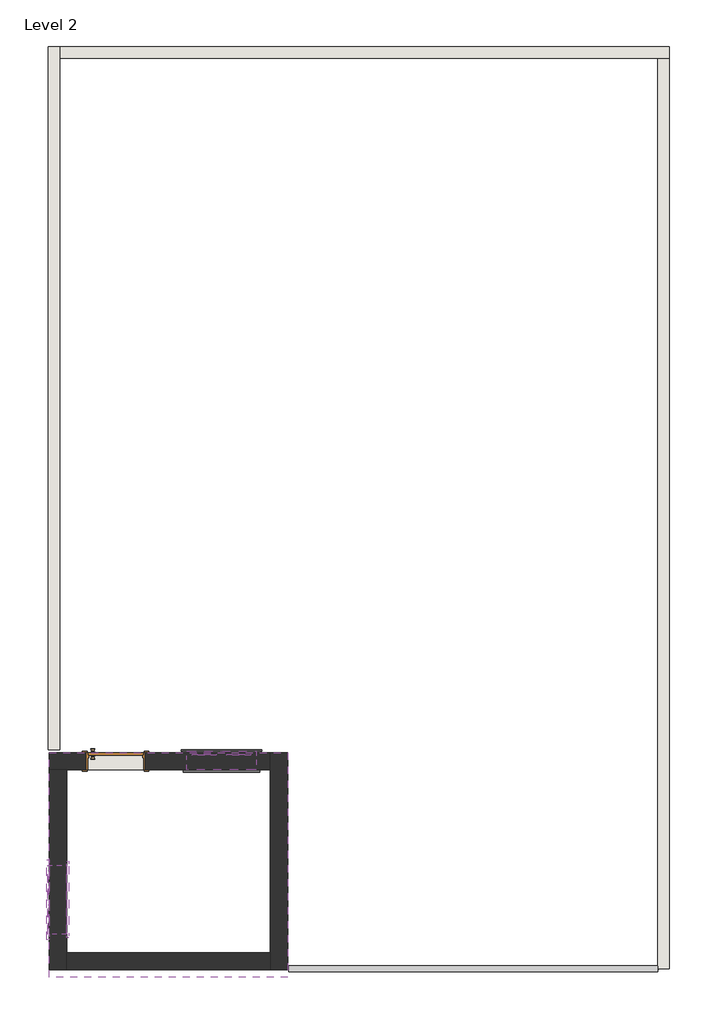
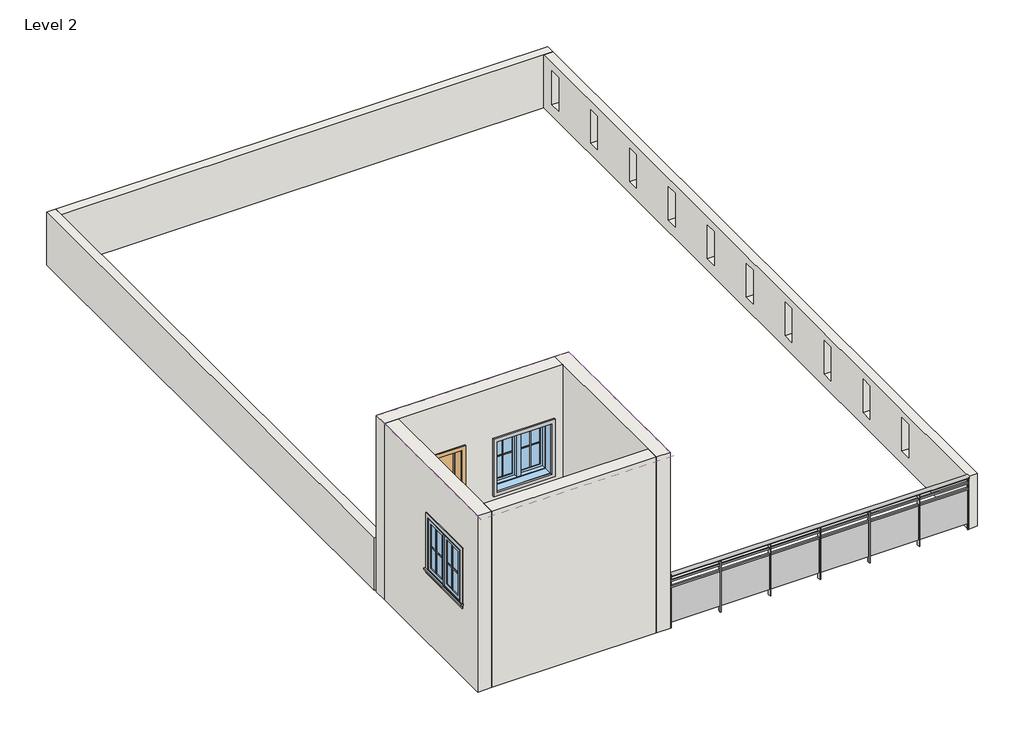
# One storey: 8 proxies, 7 walls, 2 windows, 1 covering, 1 door, 1 railing.
"""IFC4 building model written with IfcOpenShell, lengths in millimetres."""

from ifc_helpers import new_model, si_unit, point, frame, origin, place, context, project, spatial, polyline, ellipse_curve, trimmed, outline, extrude, faceted_brep, transform, mapped, element, save
from ifc_brep_helpers import plane_surface, extruded_surface, advanced_brep
from components import m_muntin_pattern_2x2_m_muntin_pattern_2x2_55460d9e, m_muntin_pattern_2x2_m_muntin_pattern_2x2_a9b7b7a9, m_trim_window_exterior_flat_with_sill_8fa486dc, m_trim_window_interior_flat_picture_frame_b6dd03a6, m_door_interior_single_flush_panel_wood_m_door_interior_542f8053, m_window_casement_double_914_x_900mm_7ae2d64b

model = new_model("IFC4")

# Units and contexts
model_context = context("Model", 3, world=origin())
ifc_project = project(units=[si_unit("LENGTHUNIT", "METRE", prefix="MILLI")], contexts=[model_context])

# Site, building, storey
site = spatial("IfcSite", under=ifc_project)
building = spatial("IfcBuilding", under=site)
storey = spatial("IfcBuildingStorey", under=building, Name="Level 2", Elevation=3048.0)

# Proxies
placement = place(None, origin())
m_muntin_pattern_2x2_m_muntin_pattern_2x2_shape = m_muntin_pattern_2x2_m_muntin_pattern_2x2_55460d9e(model_context)
element("IfcBuildingElementProxy", 1, Name="M_Muntin Pattern_2x2 : M_Muntin Pattern_2x2", ObjectType="M_Muntin Pattern_2x2 : M_Muntin Pattern_2x2", at=placement, inside=storey, context=model_context, shape_type="MappedRepresentation", body=[
    mapped(m_muntin_pattern_2x2_m_muntin_pattern_2x2_shape, transform((-3709.2004317, -3162.8938563, 4343.0929106), x_axis=(1.0, 0.0, 0.0), y_axis=(0.0, 1.0, 0.0), z_axis=(0.0, 0.0, 1.0))),
])
element("IfcBuildingElementProxy", 2, Name="M_Muntin Pattern_2x2 : M_Muntin Pattern_2x2", ObjectType="M_Muntin Pattern_2x2 : M_Muntin Pattern_2x2", at=placement, inside=storey, context=model_context, shape_type="MappedRepresentation", body=[
    mapped(m_muntin_pattern_2x2_m_muntin_pattern_2x2_shape, transform((-5746.7629317, -5323.4813563, 4402.5622211), x_axis=(0.0, 1.0, 0.0), y_axis=(-1.0, 0.0, 0.0), z_axis=(0.0, 0.0, 1.0))),
])
m_muntin_pattern_2x2_m_muntin_pattern_2x2_2_shape = m_muntin_pattern_2x2_m_muntin_pattern_2x2_a9b7b7a9(model_context)
element("IfcBuildingElementProxy", 3, Name="M_Muntin Pattern_2x2 : M_Muntin Pattern_2x2", ObjectType="M_Muntin Pattern_2x2 : M_Muntin Pattern_2x2", at=placement, inside=storey, context=model_context, shape_type="MappedRepresentation", body=[
    mapped(m_muntin_pattern_2x2_m_muntin_pattern_2x2_2_shape, transform((-3255.1754317, -3162.8938563, 4343.0929106), x_axis=(-1.0, 0.0, 0.0), y_axis=(0.0, -1.0, 0.0), z_axis=(0.0, 0.0, 1.0))),
])
element("IfcBuildingElementProxy", 4, Name="M_Muntin Pattern_2x2 : M_Muntin Pattern_2x2", ObjectType="M_Muntin Pattern_2x2 : M_Muntin Pattern_2x2", at=placement, inside=storey, context=model_context, shape_type="MappedRepresentation", body=[
    mapped(m_muntin_pattern_2x2_m_muntin_pattern_2x2_2_shape, transform((-5746.7629317, -4869.4563563, 4402.5622211), x_axis=(0.0, -1.0, 0.0), y_axis=(1.0, 0.0, 0.0), z_axis=(0.0, 0.0, 1.0))),
])
m_trim_window_exterior_flat_with_sill_shape = m_trim_window_exterior_flat_with_sill_8fa486dc(model_context)
element("IfcBuildingElementProxy", 5, Name="M_Trim-Window-Exterior-Flat : with Sill", ObjectType="M_Trim-Window-Exterior-Flat : with Sill", at=placement, inside=storey, context=model_context, shape_type="MappedRepresentation", body=[
    mapped(m_trim_window_exterior_flat_with_sill_shape, transform((-3482.1879317, -3153.3688563, 5173.2429106), x_axis=(-1.0, 0.0, 0.0), y_axis=(0.0, 0.0, 1.0), z_axis=(0.0, 1.0, 0.0))),
])
element("IfcBuildingElementProxy", 6, Name="M_Trim-Window-Exterior-Flat : with Sill", ObjectType="M_Trim-Window-Exterior-Flat : with Sill", at=placement, inside=storey, context=model_context, shape_type="MappedRepresentation", body=[
    mapped(m_trim_window_exterior_flat_with_sill_shape, transform((-5756.2879317, -5096.4688563, 5232.7122211), x_axis=(0.0, -1.0, 0.0), y_axis=(0.0, 0.0, 1.0), z_axis=(-1.0, 0.0, 0.0))),
])
m_trim_window_interior_flat_picture_frame_shape = m_trim_window_interior_flat_picture_frame_b6dd03a6(model_context)
element("IfcBuildingElementProxy", 7, Name="M_Trim-Window-Interior-Flat : Picture Frame", ObjectType="M_Trim-Window-Interior-Flat : Picture Frame", at=placement, inside=storey, context=model_context, shape_type="MappedRepresentation", body=[
    mapped(m_trim_window_interior_flat_picture_frame_shape, transform((-3482.1879317, -3381.9688563, 5173.2429106), x_axis=(1.0, 0.0, 0.0), y_axis=(0.0, 0.0, 1.0), z_axis=(0.0, -1.0, 0.0))),
])
element("IfcBuildingElementProxy", 8, Name="M_Trim-Window-Interior-Flat : Picture Frame", ObjectType="M_Trim-Window-Interior-Flat : Picture Frame", at=placement, inside=storey, context=model_context, shape_type="MappedRepresentation", body=[
    mapped(m_trim_window_interior_flat_picture_frame_shape, transform((-5527.6879317, -5096.4688563, 5232.7122211), x_axis=(0.0, 1.0, 0.0), y_axis=(0.0, 0.0, 1.0), z_axis=(1.0, 0.0, 0.0))),
])

# Covering
element("IfcCovering", 9, ObjectType="2' x 4' ACT System", at=placement, inside=storey, context=model_context, shape_type="SweptSolid", body=[
    extrude(outline(polyline([(-2605.8879317, -3153.3688563), (-2605.8879317, -6125.1688563), (-5756.2879317, -6125.1688563), (-5756.2879317, -3153.3688563), (-2605.8879317, -3153.3688563)])), frame((0.0, 0.0, 6096.0), z_axis=(0.0, 0.0, 1.0), x_axis=(1.0, 0.0, 0.0)), (0.0, 0.0, 1.0), 57.15),
])

# Door
m_door_interior_single_flush_panel_wood_m_door_interior_shape = m_door_interior_single_flush_panel_wood_m_door_interior_542f8053(model_context)
element("IfcDoor", 10, ObjectType="M_Door-Interior-Single-Flush_Panel-Wood : M_Door-Interior-Single-Flush_Panel-Wood", at=placement, inside=storey, context=model_context, shape_type="MappedRepresentation", body=[
    mapped(m_door_interior_single_flush_panel_wood_m_door_interior_shape, transform((-4879.9879317, -3264.4938563, 3200.4), x_axis=(1.0, 0.0, 0.0), y_axis=(0.0, 1.0, 0.0), z_axis=(0.0, 0.0, 1.0))),
])

# Railing
element("IfcRailing", 11, ObjectType="Glass Panel - Bottom Fill", at=placement, inside=storey, context=model_context, shape_type="SolidModel", body=[
    advanced_brep(
    [(2282.8120683, -6048.9688563, 3962.4), (2282.8120683, -5972.7688563, 3962.4), (-2593.9879317, -6048.9688563, 3962.4), (-2593.9879317, -5972.7688563, 3962.4)],
    [
        (0, 1, ellipse_curve(frame((2282.8120683, -6010.8688563, 3962.4), z_axis=(1.0, 0.0, 0.0), x_axis=(0.0, 1.0, 0.0)), 38.1, 28.575)),
        (1, 0, ellipse_curve(frame((2282.8120683, -6010.8688563, 3962.4), z_axis=(1.0, 0.0, 0.0), x_axis=(0.0, 1.0, 0.0)), 38.1, 28.575)),
        (2, 3, ellipse_curve(frame((-2593.9879317, -6010.8688563, 3962.4), z_axis=(-1.0, 0.0, 0.0), x_axis=(0.0, 1.0, 0.0)), 38.1, 28.575)),
        (3, 2, ellipse_curve(frame((-2593.9879317, -6010.8688563, 3962.4), z_axis=(-1.0, 0.0, 0.0), x_axis=(0.0, 1.0, 0.0)), 38.1, 28.575)),
        (0, 2),
        (3, 1),
    ],
    [
        plane_surface(frame((2282.8120683, -6010.8688563, 3962.4), z_axis=(1.0, 0.0, 0.0), x_axis=(0.0, -1.0, 0.0))),
        plane_surface(frame((-2593.9879317, -6010.8688563, 3962.4), z_axis=(-1.0, 0.0, 0.0), x_axis=(0.0, -1.0, 0.0))),
        extruded_surface(trimmed(ellipse_curve(frame((-2593.9879317, -6010.8688563, 3962.4), z_axis=(1.0, 0.0, 0.0), x_axis=(0.0, 1.0, 0.0)), 38.1, 28.575), [point((-2593.9879317, -6048.9688563, 3962.4))], [point((-2593.9879317, -5972.7688563, 3962.4))], True, "CARTESIAN"), (4876.8, 0.0, 0.0), 4876.8),
        extruded_surface(trimmed(ellipse_curve(frame((-2593.9879317, -6010.8688563, 3962.4), z_axis=(1.0, 0.0, 0.0), x_axis=(0.0, 1.0, 0.0)), 38.1, 28.575), [point((-2593.9879317, -5972.7688563, 3962.4))], [point((-2593.9879317, -6048.9688563, 3962.4))], True, "CARTESIAN"), (4876.8, 0.0, 0.0), 4876.8),
    ],
    [
        (0, [[1, 2]]),
        (1, [[3, 4]]),
        (2, [[-1, 5, -4, 6]]),
        (3, [[-2, -6, -3, -5]]),
    ],
),
    extrude(outline(polyline([(2282.8120683, -5998.1688563), (2282.8120683, -6023.5688563), (-2593.9879317, -6023.5688563), (-2593.9879317, -5998.1688563), (2282.8120683, -5998.1688563)])), frame((0.0, 0.0, 3848.1), z_axis=(0.0, 0.0, 1.0), x_axis=(1.0, 0.0, 0.0)), (0.0, 0.0, 1.0), 25.4),
    extrude(outline(polyline([(2282.8120683, -5998.1688563), (2282.8120683, -6023.5688563), (-2593.9879317, -6023.5688563), (-2593.9879317, -5998.1688563), (2282.8120683, -5998.1688563)])), frame((0.0, 0.0, 3746.5), z_axis=(0.0, 0.0, 1.0), x_axis=(1.0, 0.0, 0.0)), (0.0, 0.0, 1.0), 25.4),
    extrude(outline(polyline([(-1781.1879317, -6017.4040133), (-2593.9879317, -6017.4040133), (-2593.9879317, -6011.0540133), (-1781.1879317, -6011.0540133), (-1781.1879317, -6017.4040133)])), frame((0.0, 0.0, 3149.6), z_axis=(0.0, 0.0, 1.0), x_axis=(1.0, 0.0, 0.0)), (0.0, 0.0, 1.0), 596.9),
    extrude(outline(polyline([(-1774.8379317, -5985.4688563), (-1774.8379317, -6036.2688563), (-1787.5379317, -6036.2688563), (-1787.5379317, -5985.4688563), (-1774.8379317, -5985.4688563)])), frame((0.0, 0.0, 3048.0), z_axis=(0.0, 0.0, 1.0), x_axis=(1.0, 0.0, 0.0)), (0.0, 0.0, 1.0), 885.825),
    extrude(outline(polyline([(-968.3879317, -6017.4040133), (-1781.1879317, -6017.4040133), (-1781.1879317, -6011.0540133), (-968.3879317, -6011.0540133), (-968.3879317, -6017.4040133)])), frame((0.0, 0.0, 3149.6), z_axis=(0.0, 0.0, 1.0), x_axis=(1.0, 0.0, 0.0)), (0.0, 0.0, 1.0), 596.9),
    extrude(outline(polyline([(-962.0379317, -5985.4688563), (-962.0379317, -6036.2688563), (-974.7379317, -6036.2688563), (-974.7379317, -5985.4688563), (-962.0379317, -5985.4688563)])), frame((0.0, 0.0, 3048.0), z_axis=(0.0, 0.0, 1.0), x_axis=(1.0, 0.0, 0.0)), (0.0, 0.0, 1.0), 885.825),
    extrude(outline(polyline([(-155.5879317, -6017.4040133), (-968.3879317, -6017.4040133), (-968.3879317, -6011.0540133), (-155.5879317, -6011.0540133), (-155.5879317, -6017.4040133)])), frame((0.0, 0.0, 3149.6), z_axis=(0.0, 0.0, 1.0), x_axis=(1.0, 0.0, 0.0)), (0.0, 0.0, 1.0), 596.9),
    extrude(outline(polyline([(-149.2379317, -5985.4688563), (-149.2379317, -6036.2688563), (-161.9379317, -6036.2688563), (-161.9379317, -5985.4688563), (-149.2379317, -5985.4688563)])), frame((0.0, 0.0, 3048.0), z_axis=(0.0, 0.0, 1.0), x_axis=(1.0, 0.0, 0.0)), (0.0, 0.0, 1.0), 885.825),
    extrude(outline(polyline([(657.2120683, -6017.4040133), (-155.5879317, -6017.4040133), (-155.5879317, -6011.0540133), (657.2120683, -6011.0540133), (657.2120683, -6017.4040133)])), frame((0.0, 0.0, 3149.6), z_axis=(0.0, 0.0, 1.0), x_axis=(1.0, 0.0, 0.0)), (0.0, 0.0, 1.0), 596.9),
    extrude(outline(polyline([(663.5620683, -5985.4688563), (663.5620683, -6036.2688563), (650.8620683, -6036.2688563), (650.8620683, -5985.4688563), (663.5620683, -5985.4688563)])), frame((0.0, 0.0, 3048.0), z_axis=(0.0, 0.0, 1.0), x_axis=(1.0, 0.0, 0.0)), (0.0, 0.0, 1.0), 885.825),
    extrude(outline(polyline([(1470.0120683, -6017.4040133), (657.2120683, -6017.4040133), (657.2120683, -6011.0540133), (1470.0120683, -6011.0540133), (1470.0120683, -6017.4040133)])), frame((0.0, 0.0, 3149.6), z_axis=(0.0, 0.0, 1.0), x_axis=(1.0, 0.0, 0.0)), (0.0, 0.0, 1.0), 596.9),
    extrude(outline(polyline([(1476.3620683, -5985.4688563), (1476.3620683, -6036.2688563), (1463.6620683, -6036.2688563), (1463.6620683, -5985.4688563), (1476.3620683, -5985.4688563)])), frame((0.0, 0.0, 3048.0), z_axis=(0.0, 0.0, 1.0), x_axis=(1.0, 0.0, 0.0)), (0.0, 0.0, 1.0), 885.825),
    extrude(outline(polyline([(2282.8120683, -6017.4040133), (1470.0120683, -6017.4040133), (1470.0120683, -6011.0540133), (2282.8120683, -6011.0540133), (2282.8120683, -6017.4040133)])), frame((0.0, 0.0, 3149.6), z_axis=(0.0, 0.0, 1.0), x_axis=(1.0, 0.0, 0.0)), (0.0, 0.0, 1.0), 596.9),
    extrude(outline(polyline([(-2581.2879317, -6001.3438563), (-2581.2879317, -6020.3938563), (-2600.3379317, -6020.3938563), (-2600.3379317, -6001.3438563), (-2581.2879317, -6001.3438563)])), frame((0.0, 0.0, 3048.0), z_axis=(0.0, 0.0, 1.0), x_axis=(1.0, 0.0, 0.0)), (0.0, 0.0, 1.0), 885.825),
    extrude(outline(polyline([(2289.1620683, -6001.3438563), (2289.1620683, -6020.3938563), (2270.1120683, -6020.3938563), (2270.1120683, -6001.3438563), (2289.1620683, -6001.3438563)])), frame((0.0, 0.0, 3048.0), z_axis=(0.0, 0.0, 1.0), x_axis=(1.0, 0.0, 0.0)), (0.0, 0.0, 1.0), 885.825),
])

# Walls
element("IfcWall", 12, ObjectType="Generic - 6\"", at=placement, inside=storey, context=model_context, shape_type="Brep", body=[
    faceted_brep([(-5768.9879317, 6181.1311437, 3048.0), (-5768.9879317, -3115.2688563, 3048.0), (-5768.9879317, -3115.2688563, 3962.4), (-5768.9879317, 6181.1311437, 3962.4), (-5616.5879317, 6181.1311437, 3048.0), (-5616.5879317, 6181.1311437, 3962.4), (-5616.5879317, 6028.7311437, 3962.4), (-5616.5879317, -3115.2688563, 3962.4), (-5616.5879317, -3115.2688563, 3048.0), (-5616.5879317, 6028.7311437, 3048.0)], [[[0, 1, 2, 3]], [[4, 5, 6, 7, 8, 9]], [[1, 0, 4, 9, 8]], [[2, 1, 8, 7]], [[3, 2, 7, 6, 5]], [[0, 3, 5, 4]]]),
])
element("IfcWall", 13, ObjectType="Generic - 6\"", at=placement, inside=storey, context=model_context, shape_type="Brep", body=[
    faceted_brep([(2435.2120683, 6181.1311437, 3048.0), (-5616.5879317, 6181.1311437, 3048.0), (-5616.5879317, 6181.1311437, 3962.4), (2435.2120683, 6181.1311437, 3962.4), (2435.2120683, 6028.7311437, 3048.0), (2435.2120683, 6028.7311437, 3962.4), (2282.8120683, 6028.7311437, 3962.4), (-5616.5879317, 6028.7311437, 3962.4), (-5616.5879317, 6028.7311437, 3048.0), (2282.8120683, 6028.7311437, 3048.0)], [[[0, 1, 2, 3]], [[4, 5, 6, 7, 8, 9]], [[1, 0, 4, 9, 8]], [[3, 2, 7, 6, 5]], [[2, 1, 8, 7]], [[0, 3, 5, 4]]]),
])
element("IfcWall", 14, ObjectType="Generic - 6\"", at=placement, inside=storey, context=model_context, shape_type="SweptSolid", body=[
    extrude(outline(polyline([(6028.7311437, 3048.0), (-6010.8688563, 3048.0), (-6010.8688563, 3962.4), (6028.7311437, 3962.4), (6028.7311437, 3048.0)]), holes=[polyline([(-4132.8026433, 3843.4293312), (-4325.6053444, 3843.4293312), (-4325.6053444, 3260.2511305), (-4132.8026433, 3260.2511305), (-4132.8026433, 3843.4293312)]), polyline([(5800.1311437, 3823.6711308), (5607.3284426, 3823.6711308), (5607.3284426, 3240.4929301), (5800.1311437, 3240.4929301), (5800.1311437, 3823.6711308)]), polyline([(4696.471834, 3825.8664864), (4503.669133, 3825.8664864), (4503.669133, 3242.6882857), (4696.471834, 3242.6882857), (4696.471834, 3825.8664864)]), polyline([(3592.8125243, 3828.061842), (3400.0098233, 3828.061842), (3400.0098233, 3244.8836413), (3592.8125243, 3244.8836413), (3592.8125243, 3828.061842)]), polyline([(2489.1532147, 3830.2571976), (2296.3505136, 3830.2571976), (2296.3505136, 3247.0789969), (2489.1532147, 3247.0789969), (2489.1532147, 3830.2571976)]), polyline([(1385.493905, 3832.4525532), (1192.691204, 3832.4525532), (1192.691204, 3249.2743525), (1385.493905, 3249.2743525), (1385.493905, 3832.4525532)]), polyline([(281.8345953, 3834.6479088), (89.0318943, 3834.6479088), (89.0318943, 3251.4697081), (281.8345953, 3251.4697081), (281.8345953, 3834.6479088)]), polyline([(-821.8247143, 3836.8432644), (-1014.6274154, 3836.8432644), (-1014.6274154, 3253.6650637), (-821.8247143, 3253.6650637), (-821.8247143, 3836.8432644)]), polyline([(-1925.484024, 3839.03862), (-2118.286725, 3839.03862), (-2118.286725, 3255.8604193), (-1925.484024, 3255.8604193), (-1925.484024, 3839.03862)]), polyline([(-3029.1433337, 3841.2339756), (-3221.9460347, 3841.2339756), (-3221.9460347, 3258.0557749), (-3029.1433337, 3258.0557749), (-3029.1433337, 3841.2339756)])]), frame((2282.8120683, 0.0, 0.0), z_axis=(1.0, 0.0, 0.0), x_axis=(0.0, 1.0, 0.0)), (0.0, 0.0, 1.0), 152.4),
])
element("IfcWall", 15, ObjectType="Generic - 9\"", at=placement, inside=storey, context=model_context, shape_type="Brep", body=[
    faceted_brep([(-2605.8879317, -6023.5688563, 3048.0), (-2605.8879317, -3153.3688563, 3048.0), (-2605.8879317, -3153.3688563, 6096.0), (-2605.8879317, -6023.5688563, 6096.0), (-2834.4879317, -6023.5688563, 3048.0), (-2834.4879317, -6023.5688563, 6096.0), (-2834.4879317, -5794.9688563, 6096.0), (-2834.4879317, -3381.9688563, 6096.0), (-2834.4879317, -3153.3688563, 6096.0), (-2834.4879317, -3153.3688563, 3048.0), (-2834.4879317, -3381.9688563, 3048.0), (-2834.4879317, -5794.9688563, 3048.0)], [[[0, 1, 2, 3]], [[4, 5, 6, 7, 8, 9, 10, 11]], [[1, 0, 4, 11, 10, 9]], [[3, 2, 8, 7, 6, 5]], [[2, 1, 9, 8]], [[0, 3, 5, 4]]]),
])
element("IfcWall", 16, ObjectType="Generic - 9\"", at=placement, inside=storey, context=model_context, shape_type="Brep", body=[
    faceted_brep([(-2834.4879317, -3153.3688563, 3048.0), (-5756.2879317, -3153.3688563, 3048.0), (-5756.2879317, -3153.3688563, 6096.0), (-2834.4879317, -3153.3688563, 6096.0), (-4486.6879317, -3153.3688563, 3200.4), (-4486.6879317, -3153.3688563, 5225.4), (-5273.2879317, -3153.3688563, 5225.4), (-5273.2879317, -3153.3688563, 3200.4), (-3024.9879317, -3153.3688563, 5173.2429106), (-3939.3879317, -3153.3688563, 5173.2429106), (-3939.3879317, -3153.3688563, 4273.2429106), (-3024.9879317, -3153.3688563, 4273.2429106), (-5756.2879317, -3381.9688563, 3048.0), (-5527.6879317, -3381.9688563, 3048.0), (-2834.4879317, -3381.9688563, 3048.0), (-2834.4879317, -3381.9688563, 6096.0), (-5527.6879317, -3381.9688563, 6096.0), (-5756.2879317, -3381.9688563, 6096.0), (-4486.6879317, -3381.9688563, 5225.4), (-4486.6879317, -3381.9688563, 3200.4), (-5273.2879317, -3381.9688563, 3200.4), (-5273.2879317, -3381.9688563, 5225.4), (-3024.9879317, -3381.9688563, 5173.2429106), (-3024.9879317, -3381.9688563, 4273.2429106), (-3939.3879317, -3381.9688563, 4273.2429106), (-3939.3879317, -3381.9688563, 5173.2429106)], [[[0, 1, 2, 3], [4, 5, 6, 7], [8, 9, 10, 11]], [[12, 13, 14, 15, 16, 17], [18, 19, 20, 21], [22, 23, 24, 25]], [[1, 0, 14, 13, 12]], [[3, 2, 17, 16, 15]], [[2, 1, 12, 17]], [[14, 0, 3, 15]], [[4, 19, 18, 5]], [[5, 18, 21, 6]], [[6, 21, 20, 7]], [[19, 4, 7, 20]], [[23, 22, 8, 11]], [[24, 23, 11, 10]], [[25, 24, 10, 9]], [[22, 25, 9, 8]]]),
])
element("IfcWall", 17, ObjectType="Generic - 9\"", at=placement, inside=storey, context=model_context, shape_type="Brep", body=[
    faceted_brep([(-5756.2879317, -3381.9688563, 3048.0), (-5756.2879317, -6023.5688563, 3048.0), (-5756.2879317, -6023.5688563, 6096.0), (-5756.2879317, -3381.9688563, 6096.0), (-5756.2879317, -4639.2688563, 5232.7122211), (-5756.2879317, -5553.6688563, 5232.7122211), (-5756.2879317, -5553.6688563, 4332.7122211), (-5756.2879317, -4639.2688563, 4332.7122211), (-5527.6879317, -3381.9688563, 3048.0), (-5527.6879317, -3381.9688563, 6096.0), (-5527.6879317, -5794.9688563, 6096.0), (-5527.6879317, -6023.5688563, 6096.0), (-5527.6879317, -6023.5688563, 3048.0), (-5527.6879317, -5794.9688563, 3048.0), (-5527.6879317, -4639.2688563, 5232.7122211), (-5527.6879317, -4639.2688563, 4332.7122211), (-5527.6879317, -5553.6688563, 4332.7122211), (-5527.6879317, -5553.6688563, 5232.7122211)], [[[0, 1, 2, 3], [4, 5, 6, 7]], [[8, 9, 10, 11, 12, 13], [14, 15, 16, 17]], [[1, 0, 8, 13, 12]], [[3, 2, 11, 10, 9]], [[0, 3, 9, 8]], [[2, 1, 12, 11]], [[15, 14, 4, 7]], [[16, 15, 7, 6]], [[17, 16, 6, 5]], [[14, 17, 5, 4]]]),
])
element("IfcWall", 18, ObjectType="Generic - 9\"", at=placement, inside=storey, context=model_context, shape_type="SweptSolid", body=[
    extrude(outline(polyline([(-2834.4879317, -6023.5688563), (-5527.6879317, -6023.5688563), (-5527.6879317, -5794.9688563), (-2834.4879317, -5794.9688563), (-2834.4879317, -6023.5688563)])), frame((0.0, 0.0, 3048.0), z_axis=(0.0, 0.0, 1.0), x_axis=(1.0, 0.0, 0.0)), (0.0, 0.0, 1.0), 3048.0),
])

# Windows
m_window_casement_double_914_x_900mm_shape = m_window_casement_double_914_x_900mm_7ae2d64b(model_context)
element("IfcWindow", 19, ObjectType="M_Window-Casement-Double : 914 x 900mm", at=placement, inside=storey, context=model_context, shape_type="MappedRepresentation", body=[
    mapped(m_window_casement_double_914_x_900mm_shape, transform((-3482.1879317, -3267.6688563, 3373.2429106), x_axis=(1.0, 0.0, 0.0), y_axis=(0.0, 1.0, 0.0), z_axis=(0.0, 0.0, 1.0))),
])
element("IfcWindow", 20, ObjectType="M_Window-Casement-Double : 914 x 900mm", at=placement, inside=storey, context=model_context, shape_type="MappedRepresentation", body=[
    mapped(m_window_casement_double_914_x_900mm_shape, transform((-5641.9879317, -5096.4688563, 3432.7122211), x_axis=(0.0, 1.0, 0.0), y_axis=(-1.0, 0.0, 0.0), z_axis=(0.0, 0.0, 1.0))),
])

save(model, "model.ifc")

# Revit data of these elements
# Type "M_Muntin Pattern_2x2 : M_Muntin Pattern_2x2"
#   Width [instance default] = 3' - 11.24409"
#   Thickness = 0' - 0 1/2"
#   Height [instance default] = 3' - 11.24409"
#   Distance = 0' - 0 3/4"
#   Interior Material [instance default] = none
#   Exterior Material [instance default] = none
#   Default Elevation = 0
# Type "M_Trim-Window-Exterior-Flat : with Sill"
#   Trim Width = 0' - 2.3622"
#   Trim Thickness_Picture Frame = 0' - 1.1811"
#   Trim Thickness_with Sill = 0' - 0 3/4"
#   Sill Thickness = 0' - 1.1811"
#   Opening Width [instance default] = 1' - 11.62205"
#   Opening Height [instance default] = 2' - 11.43307"
#   Default Elevation = 3' - 11.24409"
#   Sill = yes
#   Picture Frame = no
#   Trim Material [instance default] = none
# Type "M_Trim-Window-Interior-Flat : Picture Frame"
#   Trim Thickness_Picture Frame = 0' - 1.1811"
#   Trim Width = 0' - 2.3622"
#   Trim Thickness_with Sill = 0' - 0.7874"
#   Sill Thickness = 0' - 1.1811"
#   Opening Width [instance default] = 1' - 11.62205"
#   Opening Height [instance default] = 2' - 11.43307"
#   Default Elevation = 3' - 11.24409"
#   Sill = no
#   Picture Frame = yes
#   Trim Material [instance default] = none
# Type "2' x 4' ACT System"
#   Assembly Code = "C3030210"
#   built-in parameter 1002203 = 1 (stored number, unit not read)
#   built-in parameter 1002202 = 1 (stored number, unit not read)
#   Layers, outside or top first: 0' - 1 5/8" "Default" (function 1); 0' - 0 5/8" "Acoustic Ceiling Tile 24 x 48" (function 5)
# Type "M_Door-Interior-Single-Flush_Panel-Wood : M_Door-Interior-Single-Flush_Panel-Wood"
#   Type Mark = "10"
#   Assembly Code = "C1020300"
#   Analytic Construction = "Wooden"
#   Thickness = 0' - 1.37795"
#   Thermal Resistance (R) = 2.5876 (h·ft²·°F)/BTU
#   Swing Angle [instance default] = 90.00°
#   Rough Width = 2' - 6.9685"
#   Rough Height = 6' - 7.72441"
#   Height = 6' - 6.74016"
#   Width = 2' - 5"
#   Heat Transfer Coefficient (U) = 0.3865 BTU/(h·ft²·°F)
#   Trim Material = Cherry
#   Panel Material = Cherry
#   Frame Material = Cherry
#   Door Handle Material = Aluminum
#   Visual Light Transmittance = 0
#   Solar Heat Gain Coefficient = 0
#   Wall Closure = (empty or 0)
#   Function = (empty or 0)
# Type "Glass Panel - Bottom Fill"
#   Assembly Code = "C2010400"
#   built-in parameter 1008612 = 0.0416667 (stored number, unit not read)
#   built-in parameter 1008611 = 0.0416667 (stored number, unit not read)
#   built-in parameter 1008609 = 0.333333 (stored number, unit not read)
#   built-in parameter 1008604 = 0.166667 (stored number, unit not read)
#   built-in parameter 1008603 = 0.166667 (stored number, unit not read)
#   Railing Height = 3' - 0"
#   built-in parameter 1008630 = 2
#   built-in parameter 1008610 = 2
#   built-in parameter 1008618 = Baluster - Square : 3/4"
# Type "Generic - 6\""
#   Assembly Code = "B2010"
#   Layers, outside or top first: 0' - 6" no material (function 1)
# Type "Generic - 9\""
#   Assembly Code = "B2010"
#   Layers, outside or top first: 0' - 9" no material (function 1)
# Type "M_Window-Casement-Double : 914 x 900mm"
#   Type Mark = "20"
#   Fire Rating = "0.5h"
#   Assembly Code = "B2020100"
#   Analytic Construction = "Double glazing - domestic"
#   Frame Extension [instance default] = 0' - 0 1/4"
#   Window Inset [instance default] = 0' - 0"
#   Wall Thickness [instance default] = 0' - 5.90551"
#   Interior Wall Closure [instance default] = 0' - 2.15551"
#   Half Width = 1' - 6"
#   Visual Light Transmittance = 0.81
#   Thermal Resistance (R) = 1.8146 (h·ft²·°F)/BTU
#   Solar Heat Gain Coefficient = 0.76
#   Rough Width = 3' - 0.59055"
#   Rough Height = 3' - 0.02362"
#   Height = 2' - 11.43307"
#   Heat Transfer Coefficient (U) = 0.5511 BTU/(h·ft²·°F)
#   Exterior Wall Closure [instance default] = 0' - 1.25197"
#   Extension Jamb [instance default] = 0' - 2.15551"
#   Default Sill Height = 2' - 11.43307"
#   Width = 3' - 0"
#   Muntin Visibility = yes
#   Interior Trim Visibility [instance default] = yes
#   Exterior Trim Visibility [instance default] = yes
#   Extension Jamb Visibility [instance default] = yes
#   Interior Trim Material = Wood - Stained
#   Muntin Pattern = M_Muntin Pattern_2x2 : M_Muntin Pattern_2x2
#   Interior Trim = M_Trim-Window-Interior-Flat : Picture Frame
#   Interior Frame Material = Wood - Stained
#   Glass Panel Material = Glass
#   Exterior Trim Material = Clad - White
#   Exterior Trim = M_Trim-Window-Exterior-Flat : with Sill
#   Exterior Frame Material = Clad - White
#   Wall Closure = (empty or 0)
# Elements 1, 2, 3, 4 (IfcBuildingElementProxy, "M_Muntin Pattern_2x2 : M_Muntin Pattern_2x2")
#   Width = 1' - 0 5/8"
#   Height = 2' - 5.93307"
#   Interior Material = Wood - Stained
#   Exterior Material = Clad - White
#   Phase Created = New Construction
#   Materials on its faces: "Clad - White", "Wood - Stained"
# Elements 5, 6 (IfcBuildingElementProxy, "M_Trim-Window-Exterior-Flat : with Sill")
#   Opening Width = 3' - 0"
#   Opening Height = 2' - 11.43307"
#   Trim Material = Clad - White
#   Phase Created = New Construction
#   Materials on its faces: "Clad - White"
# Elements 7, 8 (IfcBuildingElementProxy, "M_Trim-Window-Interior-Flat : Picture Frame")
#   Opening Width = 3' - 0"
#   Opening Height = 2' - 11.43307"
#   Trim Material = Wood - Stained
#   Phase Created = New Construction
#   Materials on its faces: "Wood - Stained"
# Element 9 (IfcCovering, "2' x 4' ACT System")
#   Height Offset From Level = 10' - 0"
#   Phase Created = New Construction
#   Materials on its faces: "Acoustic Ceiling Tile 24 x 48", "Default"
# Element 10 (IfcDoor, "M_Door-Interior-Single-Flush_Panel-Wood : M_Door-Interior-Single-Flush_Panel-Wood")
#   Swing Angle = 90.00°
#   Phase Created = New Construction
#   Materials on its faces: "Cherry", "Aluminum"
# Element 11 (IfcRailing, "Glass Panel - Bottom Fill")
#   Phase Created = New Construction
#   Materials on its faces: "Glass"
# Elements 12, 13, 14 (IfcWall, "Generic - 6\"")
#   Top Offset = 0' - 0"
#   Base Offset = 0' - 0"
#   Unconnected Height = 3' - 0"
#   wall height = 3' - 0"
#   Phase Created = New Construction
#   Base Constraint = Level 2
#   Materials on its faces: "Default Wall", "Brick, Common"
# Elements 15, 16, 17 (IfcWall, "Generic - 9\"")
#   Top Offset = 0' - 0"
#   Base Offset = 0' - 0"
#   Unconnected Height = 10' - 0"
#   wall height = 10' - 0"
#   Phase Created = New Construction
#   Base Constraint = Level 2
#   Materials on its faces: "Default Wall", "Brick, Common"
# Element 18 (IfcWall, "Generic - 9\"")
#   Top Offset = 0' - 0"
#   Base Offset = 0' - 0"
#   Unconnected Height = 10' - 0"
#   wall height = 10' - 0"
#   Phase Created = New Construction
#   Base Constraint = Level 2
#   Materials on its faces: "Default Wall", "Parking Stripe"
# Element 19 (IfcWindow, "M_Window-Casement-Double : 914 x 900mm")
#   Mark = "8"
#   Window Inset = 0' - 0"
#   Interior Wall Closure = 0' - 2.15551"
#   Frame Extension = 0' - 0 1/4"
#   Exterior Wall Closure = 0' - 1.25197"
#   Interior Trim Visibility = yes
#   Exterior Trim Visibility = yes
#   Phase Created = New Construction
#   Materials on its faces: "Wood - Stained", "Glass", "Clad - White"
# Element 20 (IfcWindow, "M_Window-Casement-Double : 914 x 900mm")
#   Mark = "9"
#   Window Inset = 0' - 0"
#   Interior Wall Closure = 0' - 2.15551"
#   Frame Extension = 0' - 0 1/4"
#   Exterior Wall Closure = 0' - 1.25197"
#   Interior Trim Visibility = yes
#   Exterior Trim Visibility = yes
#   Phase Created = New Construction
#   Materials on its faces: "Wood - Stained", "Glass", "Clad - White"
# Materials
#   "Default": colour RGB 127 127 127, transparency 0, Cost = 0
#   "Acoustic Ceiling Tile 24 x 48": class "Generic", colour RGB 229 229 229, transparency 0, Description = "Acoustic Ceiling Tile 24 x 48", Cost = 0
#   "Cherry": class "Wood", colour RGB 226 177 128, transparency 0, Description = "Prunus Serotina", Cost = 0
#   "Aluminum": class "Metal", colour RGB 247 247 247, transparency 0, Description = "Aluminum 6061", Cost = 0
#   "Wood - Stained": class "Wood", colour RGB 224 178 126, transparency 0, Cost = 0
#   "Glass": class "Glass", colour RGB 0 128 192, transparency 0.75, Description = "Soda Lime Glass", Cost = 0
#   "Clad - White": class "Wood", colour RGB 242 242 238, transparency 0, Cost = 0
#   "Default Wall": colour RGB 128 128 128, transparency 0, Cost = 0
#   "Brick, Common": class "Masonry", colour RGB 170 98 104, transparency 0, Description = "Common brick", Cost = 0
#   "Parking Stripe": class "Paint", colour RGB 250 250 91, transparency 0, Cost = 0
